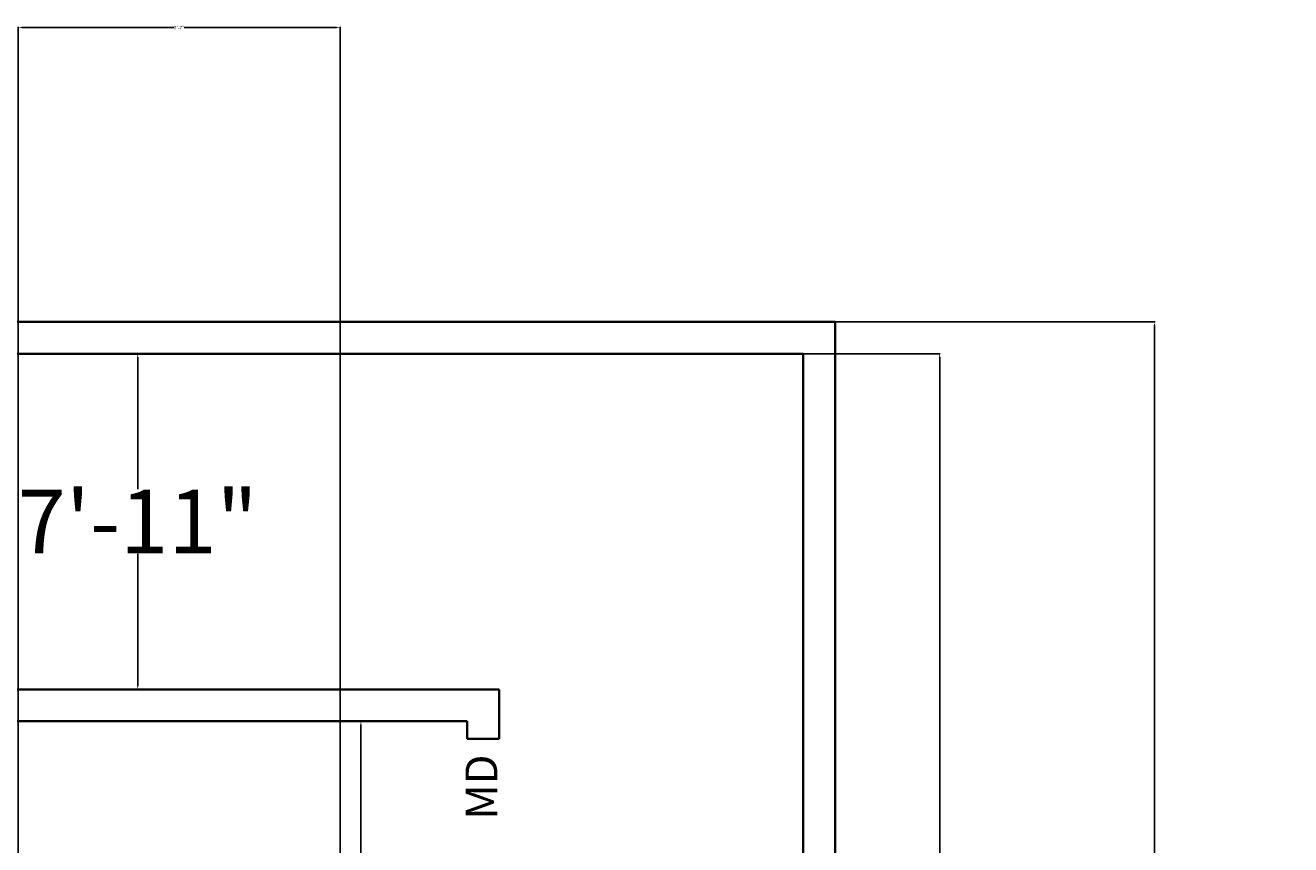
# Model space of a CAD drawing. Units: inches. Extents: x -2189 to 546, y 945 to 2684.
# Tile 9 of 10: x -492 to -134, y 2452 to 2684. Entities that reach past the tile are written whole.
import ezdxf

# ---------------------------------------------------------------- set-up
doc = ezdxf.new("R2010")
doc.units = ezdxf.units.IN
doc.header["$MEASUREMENT"] = 0
for name, color, linetype, lineweight in [('A-ANNO-DIMS', 2, 'Continuous', 13), ('A-ANNO-TEXT', 7, 'Continuous', 18), ('A-WALL', 7, 'Continuous', 35)]:
    doc.layers.add(name, color=color, linetype=linetype, lineweight=lineweight)
doc.styles.get("Standard").update_dxf_attribs({"font": 'arial.ttf'})
doc.dimstyles.get("Standard").update_dxf_attribs({"dimtxt": 1, "dimasz": 1, "dimexe": 0.18, "dimexo": 0.0625, "dimgap": 0.09, "dimtad": 0, "dimtih": 1, "dimtoh": 1, "dimdec": 0, "dimzin": 0, "dimdsep": 46, "dimlunit": 3, "dimtxsty": 'Standard', "dimcen": 0.09, "dimadec": 0, "dimazin": 0, "dimtfac": 1, "dimtdec": 0, "dimtofl": 0, "dimtmove": 0, "dimatfit": 3, "dimfxl": 1, "dimtolj": 1, "dimtzin": 0, "dimarcsym": 0})

# ---------------------------------------------------------------- blocks, each defined once
blk = doc.blocks.new('*D78')
at = {"layer": 'A-ANNO-DIMS', "color": 0, "lineweight": -2, "transparency": 16777216}
for p, q in [((-366.84, 2487.17), (-397.04, 2487.17)), ((-396.86, 2486.17), (-396.86, 2443.86)), ((-396.86, 2392.17), (-396.86, 2434.49)), ((-366.84, 2391.17), (-397.04, 2391.17))]:
    blk.add_line(p, q, dxfattribs=at)
at = {"layer": 'A-ANNO-DIMS', "color": 0, "transparency": 16777216}
for points in [[(-397.03, 2486.17), (-396.7, 2486.17), (-396.86, 2487.17)], [(-397.03, 2392.17), (-396.7, 2392.17), (-396.86, 2391.17)]]:
    blk.add_solid(points, dxfattribs=at)
at = {"layer": 'Defpoints', "color": 0, "transparency": 16777216}
for p in [(-396.86, 2487.17), (-366.78, 2487.17), (-366.78, 2391.17)]:
    blk.add_point(p, dxfattribs=at)
at = {"layer": 'A-ANNO-DIMS', "color": 0, "transparency": 16777216, "insert": (-396.86, 2439.17), "char_height": 1, "attachment_point": 5}
blk.add_mtext("\\A1;{\\H9x;8'}", dxfattribs=at)
blk = doc.blocks.new('*D79')
at = {"layer": 'A-ANNO-DIMS', "color": 0, "lineweight": -2, "transparency": 16777216}
for p, q in [((-262.72, 2600.17), (-172.26, 2600.17)), ((-172.44, 2599.17), (-172.44, 1833.96)), ((-172.44, 1050.17), (-172.44, 1815.39)), ((-262.72, 1049.17), (-172.26, 1049.17))]:
    blk.add_line(p, q, dxfattribs=at)
at = {"layer": 'A-ANNO-DIMS', "color": 0, "transparency": 16777216}
for points in [[(-172.6, 2599.17), (-172.27, 2599.17), (-172.44, 2600.17)], [(-172.6, 1050.17), (-172.27, 1050.17), (-172.44, 1049.17)]]:
    blk.add_solid(points, dxfattribs=at)
at = {"layer": 'Defpoints', "color": 0, "transparency": 16777216}
for p in [(-262.78, 2600.17), (-172.44, 2600.17), (-262.78, 1049.17)]:
    blk.add_point(p, dxfattribs=at)
at = {"layer": 'A-ANNO-DIMS', "color": 0, "transparency": 16777216, "insert": (-172.44, 1824.67), "char_height": 1, "attachment_point": 5}
blk.add_mtext('\\A1;{\\H18x;129\'-3"}', dxfattribs=at)
blk = doc.blocks.new('*D80')
at = {"layer": 'A-ANNO-DIMS', "color": 0, "lineweight": -2, "transparency": 16777216}
for p, q in [((-271.72, 2591.17), (-233.01, 2591.17)), ((-233.19, 2590.17), (-233.19, 1833.95)), ((-233.19, 1059.17), (-233.19, 1815.39)), ((-271.72, 1058.17), (-233.01, 1058.17))]:
    blk.add_line(p, q, dxfattribs=at)
at = {"layer": 'A-ANNO-DIMS', "color": 0, "transparency": 16777216}
for points in [[(-233.36, 2590.17), (-233.03, 2590.17), (-233.19, 2591.17)], [(-233.36, 1059.17), (-233.03, 1059.17), (-233.19, 1058.17)]]:
    blk.add_solid(points, dxfattribs=at)
at = {"layer": 'Defpoints', "color": 0, "transparency": 16777216}
for p in [(-271.78, 2591.17), (-233.19, 2591.17), (-271.78, 1058.17)]:
    blk.add_point(p, dxfattribs=at)
at = {"layer": 'A-ANNO-DIMS', "color": 0, "transparency": 16777216, "insert": (-233.19, 1824.67), "char_height": 1, "attachment_point": 5}
blk.add_mtext('\\A1;{\\H18x;127\'-9"}', dxfattribs=at)
blk = doc.blocks.new('*D84')
at = {"layer": 'A-ANNO-DIMS', "color": 0, "lineweight": -2, "transparency": 16777216}
for p, q in [((-452.79, 2591.17), (-460.17, 2591.17)), ((-459.99, 2590.17), (-459.99, 2552.8)), ((-459.99, 2497.17), (-459.99, 2534.55)), ((-452.79, 2496.17), (-460.17, 2496.17))]:
    blk.add_line(p, q, dxfattribs=at)
at = {"layer": 'A-ANNO-DIMS', "color": 0, "transparency": 16777216}
for points in [[(-460.16, 2590.17), (-459.83, 2590.17), (-459.99, 2591.17)], [(-460.16, 2497.17), (-459.83, 2497.17), (-459.99, 2496.17)]]:
    blk.add_solid(points, dxfattribs=at)
at = {"layer": 'Defpoints', "color": 0, "transparency": 16777216}
for p in [(-452.73, 2591.17), (-459.99, 2496.17), (-452.73, 2496.17)]:
    blk.add_point(p, dxfattribs=at)
at = {"layer": 'A-ANNO-DIMS', "color": 0, "transparency": 16777216, "insert": (-459.99, 2543.67), "char_height": 1, "attachment_point": 5}
blk.add_mtext('\\A1;{\\H18x;7\'-11"}', dxfattribs=at)
blk = doc.blocks.new('*D104')
at = {"layer": 'A-ANNO-DIMS', "color": 0, "lineweight": -2, "transparency": 16777216}
for p, q in [((-493.78, 1873.24), (-493.78, 2683.65)), ((-492.78, 2683.47), (-449.69, 2683.47)), ((-403.78, 2683.47), (-446.86, 2683.47)), ((-402.78, 1873.24), (-402.78, 2683.65))]:
    blk.add_line(p, q, dxfattribs=at)
at = {"layer": 'A-ANNO-DIMS', "color": 0, "transparency": 16777216}
for points in [[(-492.78, 2683.64), (-492.78, 2683.31), (-493.78, 2683.47)], [(-403.78, 2683.64), (-403.78, 2683.31), (-402.78, 2683.47)]]:
    blk.add_solid(points, dxfattribs=at)
at = {"layer": 'Defpoints', "color": 0, "transparency": 16777216}
for p in [(-402.78, 2683.47), (-493.78, 1873.17), (-402.78, 1873.17)]:
    blk.add_point(p, dxfattribs=at)
at = {"layer": 'A-ANNO-DIMS', "color": 0, "transparency": 16777216, "insert": (-448.28, 2683.47), "char_height": 1, "attachment_point": 5}
blk.add_mtext('\\A1;7\'-7"', dxfattribs=at)

msp = doc.modelspace()

# ---------------------------------------------------------------- linework, layer by layer
at = {"layer": 'A-WALL'}
for p, q in [((-829.78, 2600.17), (-262.78, 2600.17)), ((-262.78, 2600.17), (-262.78, 1049.17)), ((-820.78, 2591.17), (-271.78, 2591.17)), ((-271.78, 2591.17), (-271.78, 1058.17)), ((-357.78, 2496.17), (-755.78, 2496.17)), ((-357.78, 2482.17), (-357.78, 2496.17)), ((-366.78, 2487.17), (-690.78, 2487.17)), ((-366.78, 2482.17), (-366.78, 2487.17)), ((-366.78, 2482.17), (-357.78, 2482.17))]:
    msp.add_line(p, q, dxfattribs=at)

# ---------------------------------------------------------------- texts
at = {"layer": 'A-ANNO-TEXT', "insert": (-367.28, 2459.31), "char_height": 9, "attachment_point": 1, "rotation": 90}
msp.add_mtext_dynamic_manual_height_columns('MD', width=16.482, gutter_width=1, heights=[0], dxfattribs=at)

# ---------------------------------------------------------------- dimensions: what is measured, and where the dimension line sits
at = {"layer": 'A-ANNO-DIMS'}
dim = msp.add_linear_dim(base=(-402.78, 2683.47), p1=(-493.78, 1873.17), p2=(-402.78, 1873.17), dimstyle='Standard', override={"dimdec": 1, "dimlfac": 1, "dimrnd": 0, "dimzin": 1, "dimdsep": 46, "dimlunit": 4, "dimfrac": 2}, dxfattribs=at)
dim.commit()
dim.dimension.update_dxf_attribs({"geometry": '*D104', "text_midpoint": (-448.28, 2683.47)})
for base, p1, p2, text, picture, middle in [((-172.44, 2600.17), (-262.78, 1049.17), (-262.78, 2600.17), '{\\H18x;<>}', '*D79', (-172.44, 1824.67)), ((-459.99, 2496.17), (-452.73, 2591.17), (-452.73, 2496.17), '{\\H18x;<>}', '*D84', (-459.99, 2543.67)), ((-233.19, 2591.17), (-271.78, 1058.17), (-271.78, 2591.17), '{\\H18x;<>}', '*D80', (-233.19, 1824.67)), ((-396.86, 2487.17), (-366.78, 2391.17), (-366.78, 2487.17), '{\\H9x;<>}', '*D78', (-396.86, 2439.17))]:
    dim = msp.add_linear_dim(base=base, p1=p1, p2=p2, angle=90, text=text, dimstyle='Standard', override={"dimclrd": 0, "dimclre": 0, "dimclrt": 0}, dxfattribs=at)
    dim.commit()
    dim.dimension.update_dxf_attribs({"geometry": picture, "text_midpoint": middle})

doc.saveas('drawing.dxf')
